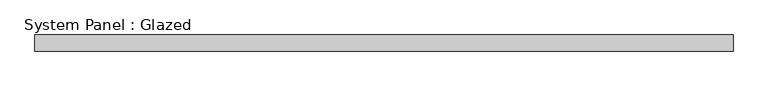
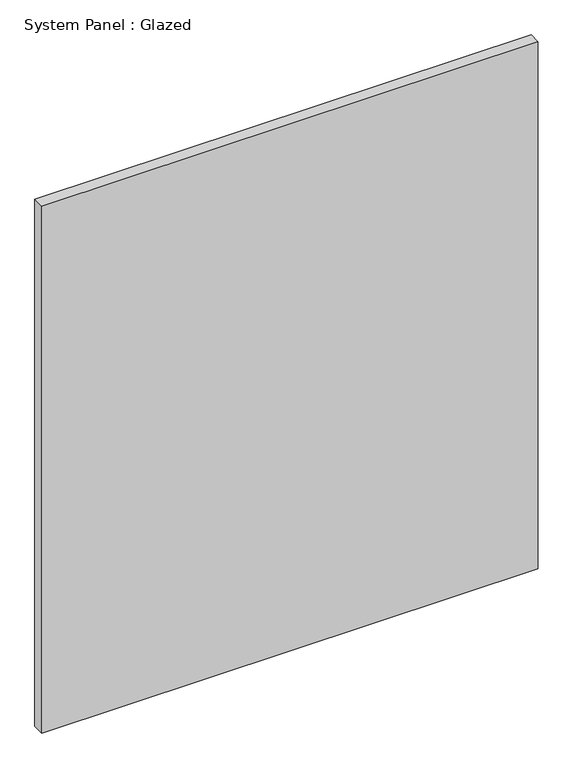
"""IFC4 building model written with IfcOpenShell, lengths in millimetres: plate geometry, System Panel : Glazed."""

from ifc_helpers import new_model, si_unit, origin, origin_with_axes, place, context, project, spatial, polyline, outline, extrude, source, transform, mapped, element, save


def system_panel_glazed_99f7726d(model_context):
    return source(origin(), model_context, "Body", "SweptSolid", [
        extrude(outline(polyline([(534.4583334, 19.05), (-534.4583334, 19.05), (-534.4583334, 44.45), (534.4583334, 44.45), (534.4583334, 19.05)])), origin_with_axes(), (0.0, 0.0, 1.0), 1198.6188597),
    ])


if __name__ == "__main__":
    model = new_model("IFC4")
    model_context = context("Model", 3, world=origin())
    ifc_project = project(units=[si_unit("LENGTHUNIT", "METRE", prefix="MILLI")], contexts=[model_context])
    site = spatial("IfcSite", under=ifc_project)
    building = spatial("IfcBuilding", under=site)
    placement = place(None, origin())
    system_panel_glazed_shape = system_panel_glazed_99f7726d(model_context)
    element("IfcPlate", 1, ObjectType="System Panel : Glazed", at=placement, inside=building, context=model_context, shape_type="MappedRepresentation", body=[
        mapped(system_panel_glazed_shape, transform((0.0, 0.0, 0.0), x_axis=(1.0, 0.0, 0.0), y_axis=(0.0, 1.0, 0.0), z_axis=(0.0, 0.0, 1.0))),
    ])
    save(model, "model.ifc")

# Revit data of these elements
# Type "System Panel : Glazed"
#   Construction Type Id = "GSP4R"
#   Analytic Construction = "1/8 in Pilkington single glazing"
#   Visual Light Transmittance = 0.9
#   Solar Heat Gain Coefficient = 0.86
#   Heat Transfer Coefficient (U) = 1.18115 BTU/(h·ft²·°F)
#   Define Thermal Properties by = 1
# Element 1 (IfcPlate, "System Panel : Glazed")
#   Materials on its faces: "Glass"
# Materials
#   "Glass": class "Glass", colour RGB 0 128 192, transparency 0.75, Description = "Soda Lime Glass", Cost = 0
